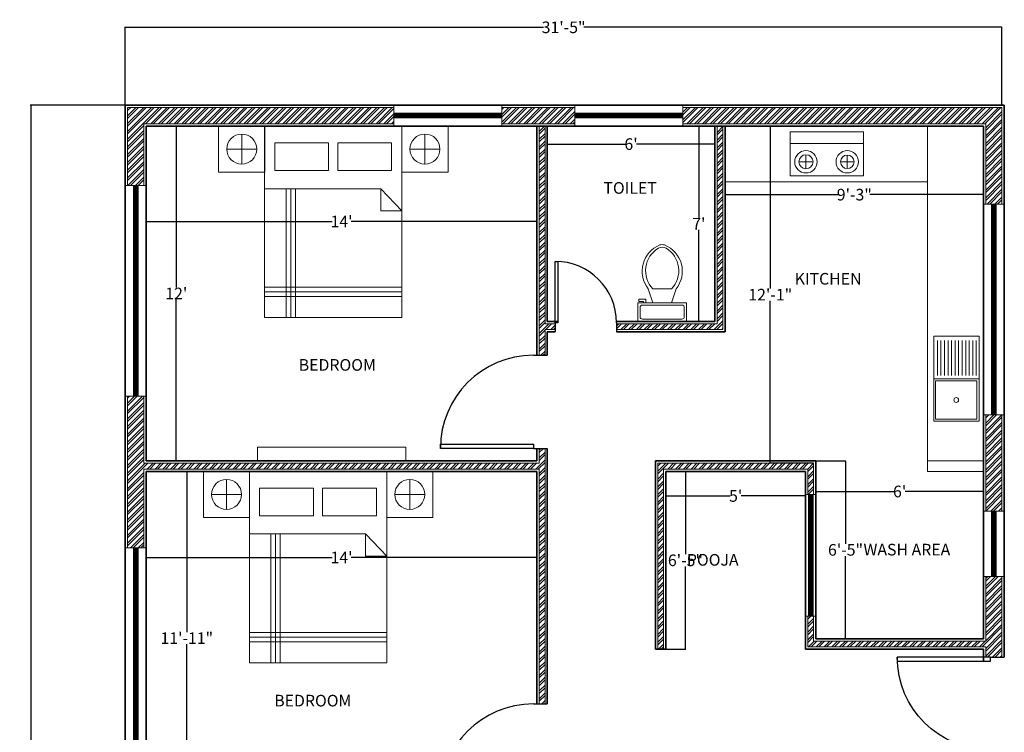
# Model space of a CAD drawing. Units: inches. Extents: x 210 to 633, y 286 to 1043.
# Tile 3 of 3: x 210 to 633, y 736 to 1043. Entities that reach past the tile are written whole.
import ezdxf

# ---------------------------------------------------------------- set-up
doc = ezdxf.new("R2010")
doc.units = ezdxf.units.IN
doc.header["$MEASUREMENT"] = 0
for name, color, linetype, lineweight in [('A-ANNO-DIMS', 170, 'Continuous', 18), ('A-AREA-IDEN', 7, 'Continuous', 25), ('A-DOOR', 4, 'Continuous', 25), ('A-EQPM', 210, 'Continuous', 18), ('A-FLOR-CBNT', 210, 'Continuous', 20), ('A-FLOR-FIXT', 210, 'Continuous', 18), ('A-FLOR-FIXT-PATT', 210, 'Continuous', 13), ('A-GLAZ-PATT', 130, 'Continuous', 13), ('A-WALL-PATT', 35, 'Continuous', 13), ('fur', 210, 'Continuous', 18), ('wall', 10, 'Continuous', 35), ('wind', 130, 'Continuous', 18)]:
    doc.layers.add(name, color=color, linetype=linetype, lineweight=lineweight)
doc.styles.get("Standard").update_dxf_attribs({"font": 'arial.ttf'})
doc.dimstyles.get("Standard").update_dxf_attribs({"dimtxt": 5, "dimasz": 0.18, "dimexe": 0.18, "dimexo": 0.0625, "dimgap": 0.09, "dimtad": 0, "dimtih": 1, "dimtoh": 1, "dimdec": 0, "dimzin": 0, "dimdsep": 46, "dimlunit": 4, "dimtxsty": 'Standard', "dimcen": 0.09, "dimadec": 0, "dimazin": 0, "dimtfac": 1, "dimtdec": 0, "dimtofl": 0, "dimtmove": 0, "dimatfit": 3, "dimfxl": 1, "dimtolj": 1, "dimtzin": 0, "dimarcsym": 0})

# ---------------------------------------------------------------- blocks, each defined once
blk = doc.blocks.new('*U2')
for p, q in [((0, 0), (0, -6)), ((40, 0), (40, -6))]:
    blk.add_line(p, q)
blk.add_lwpolyline([(0, 0), (0, 40), (1.75, 40), (1.75, 0)], close=True)
blk.add_arc((0, 0), 40, 0, 90)
blk = doc.blocks.new('*U4')
for p, q in [((9.5, -6), (9.5, -2)), ((-8, -8.5), (-8, -8)), ((-7, -8), (-7, -9.5)), ((-4, -8), (-6, -14)), ((4, -8), (6, -14)), ((-10, -8.5), (-8, -8.5)), ((-10, -9.5), (-10, -8.5)), ((-7, -9.5), (-10, -9.5)), ((4, -14), (-4, -14))]:
    blk.add_line(p, q)
blk.add_lwpolyline([(10.5, -8), (10.5, 0), (-10.5, 0), (-10.5, -8)], close=True)
for points in [[(-9.5, -2), (-9.5, -6)], [(8.5, -1), (-8.5, -1)], [(-8.5, -7), (8.5, -7)]]:
    blk.add_lwpolyline(points)
for centre, radius, start, end in [((-8.62, -1.88), 0.884, 81.8699, 188.1301), ((8.62, -1.88), 0.884, 351.8699, 98.1301), ((-8.62, -6.12), 0.884, 171.8699, 278.1301), ((8.62, -6.12), 0.884, 261.8699, 8.1301), ((3.52, -21.58), 12.17, 141.4691, 247.9714), ((4.2, -21.82), 11.33, 136.3677, 238.9468), ((-3.52, -21.58), 12.17, 292.0284, 38.5307), ((-4.2, -21.82), 11.33, 301.053, 43.6321), ((0, -27.88), 4, 245.7318, 294.2682), ((0, -29), 4, 254.8605, 285.1395)]:
    blk.add_arc(centre, radius, start, end)
blk = doc.blocks.new('*D9')
at = {"layer": 'A-ANNO-DIMS', "color": 0, "lineweight": -2, "transparency": 16777216}
for p, q in [((264.37, 996.96), (264.37, 955.79)), ((432.37, 996.96), (432.37, 955.79)), ((264.55, 955.97), (344.28, 955.97)), ((432.19, 955.97), (352.47, 955.97))]:
    blk.add_line(p, q, dxfattribs=at)
at = {"layer": 'A-ANNO-DIMS', "color": 0, "transparency": 16777216}
for points in [[(264.55, 956), (264.55, 955.94), (264.37, 955.97)], [(432.19, 956), (432.19, 955.94), (432.37, 955.97)]]:
    blk.add_solid(points, dxfattribs=at)
at = {"layer": 'Defpoints', "color": 0, "transparency": 16777216}
for p in [(264.37, 997.02), (432.37, 997.02), (432.37, 955.97)]:
    blk.add_point(p, dxfattribs=at)
at = {"layer": 'A-ANNO-DIMS', "color": 0, "transparency": 16777216, "insert": (348.37, 955.97), "char_height": 5, "attachment_point": 5}
blk.add_mtext("\\A1;14'", dxfattribs=at)
blk = doc.blocks.new('*D10')
at = {"layer": 'A-ANNO-DIMS', "color": 0, "lineweight": -2, "transparency": 16777216}
for p, q in [((264.44, 997.02), (277.51, 997.02)), ((277.33, 996.84), (277.33, 927.62)), ((277.33, 853.2), (277.33, 922.42)), ((264.44, 853.02), (277.51, 853.02))]:
    blk.add_line(p, q, dxfattribs=at)
at = {"layer": 'A-ANNO-DIMS', "color": 0, "transparency": 16777216}
for points in [[(277.3, 996.84), (277.36, 996.84), (277.33, 997.02)], [(277.3, 853.2), (277.36, 853.2), (277.33, 853.02)]]:
    blk.add_solid(points, dxfattribs=at)
at = {"layer": 'Defpoints', "color": 0, "transparency": 16777216}
for p in [(264.37, 997.02), (277.33, 997.02), (264.37, 853.02)]:
    blk.add_point(p, dxfattribs=at)
at = {"layer": 'A-ANNO-DIMS', "color": 0, "transparency": 16777216, "insert": (277.33, 925.02), "char_height": 5, "attachment_point": 5}
blk.add_mtext("\\A1;12'", dxfattribs=at)
blk = doc.blocks.new('*D11')
at = {"layer": 'A-ANNO-DIMS', "color": 0, "lineweight": -2, "transparency": 16777216}
for p, q in [((436.87, 996.96), (436.87, 989.09)), ((508.87, 996.96), (508.87, 989.09)), ((437.05, 989.27), (470.47, 989.27)), ((508.69, 989.27), (475.28, 989.27))]:
    blk.add_line(p, q, dxfattribs=at)
at = {"layer": 'A-ANNO-DIMS', "color": 0, "transparency": 16777216}
for points in [[(437.05, 989.3), (437.05, 989.24), (436.87, 989.27)], [(508.69, 989.3), (508.69, 989.24), (508.87, 989.27)]]:
    blk.add_solid(points, dxfattribs=at)
at = {"layer": 'Defpoints', "color": 0, "transparency": 16777216}
for p in [(436.87, 997.02), (508.87, 997.02), (508.87, 989.27)]:
    blk.add_point(p, dxfattribs=at)
at = {"layer": 'A-ANNO-DIMS', "color": 0, "transparency": 16777216, "insert": (472.87, 989.27), "char_height": 5, "attachment_point": 5}
blk.add_mtext("\\A1;6'", dxfattribs=at)
blk = doc.blocks.new('*D12')
at = {"layer": 'A-ANNO-DIMS', "color": 0, "lineweight": -2, "transparency": 16777216}
for p, q in [((508.81, 997.02), (501.82, 997.02)), ((502, 996.84), (502, 957.61)), ((502, 913.2), (502, 952.43)), ((508.81, 913.02), (501.82, 913.02))]:
    blk.add_line(p, q, dxfattribs=at)
at = {"layer": 'A-ANNO-DIMS', "color": 0, "transparency": 16777216}
for points in [[(501.97, 996.84), (502.03, 996.84), (502, 997.02)], [(501.97, 913.2), (502.03, 913.2), (502, 913.02)]]:
    blk.add_solid(points, dxfattribs=at)
at = {"layer": 'Defpoints', "color": 0, "transparency": 16777216}
for p in [(502, 997.02), (508.87, 997.02), (508.87, 913.02)]:
    blk.add_point(p, dxfattribs=at)
at = {"layer": 'A-ANNO-DIMS', "color": 0, "transparency": 16777216, "insert": (502, 955.02), "char_height": 5, "attachment_point": 5}
blk.add_mtext("\\A1;7'", dxfattribs=at)
blk = doc.blocks.new('*D13')
at = {"layer": 'A-ANNO-DIMS', "color": 0, "lineweight": -2, "transparency": 16777216}
for p, q in [((513.37, 996.96), (513.37, 967.35)), ((624.37, 996.96), (624.37, 967.35)), ((513.55, 967.53), (562.14, 967.53)), ((624.19, 967.53), (575.61, 967.53))]:
    blk.add_line(p, q, dxfattribs=at)
at = {"layer": 'A-ANNO-DIMS', "color": 0, "transparency": 16777216}
for points in [[(513.55, 967.56), (513.55, 967.5), (513.37, 967.53)], [(624.19, 967.56), (624.19, 967.5), (624.37, 967.53)]]:
    blk.add_solid(points, dxfattribs=at)
at = {"layer": 'Defpoints', "color": 0, "transparency": 16777216}
for p in [(513.37, 997.02), (624.37, 997.02), (624.37, 967.53)]:
    blk.add_point(p, dxfattribs=at)
at = {"layer": 'A-ANNO-DIMS', "color": 0, "transparency": 16777216, "insert": (568.87, 967.53), "char_height": 5, "attachment_point": 5}
blk.add_mtext('\\A1;9\'-3"', dxfattribs=at)
blk = doc.blocks.new('*D14')
at = {"layer": 'A-ANNO-DIMS', "color": 0, "lineweight": -2, "transparency": 16777216}
for p, q in [((551.31, 997.02), (532.55, 997.02)), ((532.73, 996.84), (532.73, 927.12)), ((532.73, 852.2), (532.73, 921.92)), ((551.31, 852.02), (532.55, 852.02))]:
    blk.add_line(p, q, dxfattribs=at)
at = {"layer": 'A-ANNO-DIMS', "color": 0, "transparency": 16777216}
for points in [[(532.7, 996.84), (532.76, 996.84), (532.73, 997.02)], [(532.7, 852.2), (532.76, 852.2), (532.73, 852.02)]]:
    blk.add_solid(points, dxfattribs=at)
at = {"layer": 'Defpoints', "color": 0, "transparency": 16777216}
for p in [(532.73, 997.02), (551.37, 997.02), (551.37, 852.02)]:
    blk.add_point(p, dxfattribs=at)
at = {"layer": 'A-ANNO-DIMS', "color": 0, "transparency": 16777216, "insert": (532.73, 924.52), "char_height": 5, "attachment_point": 5}
blk.add_mtext('\\A1;12\'-1"', dxfattribs=at)
blk = doc.blocks.new('*D15')
at = {"layer": 'A-ANNO-DIMS', "color": 0, "lineweight": -2, "transparency": 16777216}
for p, q in [((487.87, 848.46), (487.87, 837.78)), ((547.87, 848.46), (547.87, 837.78)), ((488.05, 837.96), (515.48, 837.96)), ((547.69, 837.96), (520.26, 837.96))]:
    blk.add_line(p, q, dxfattribs=at)
at = {"layer": 'A-ANNO-DIMS', "color": 0, "transparency": 16777216}
for points in [[(488.05, 837.99), (488.05, 837.93), (487.87, 837.96)], [(547.69, 837.99), (547.69, 837.93), (547.87, 837.96)]]:
    blk.add_solid(points, dxfattribs=at)
at = {"layer": 'Defpoints', "color": 0, "transparency": 16777216}
for p in [(487.87, 848.52), (547.87, 848.52), (547.87, 837.96)]:
    blk.add_point(p, dxfattribs=at)
at = {"layer": 'A-ANNO-DIMS', "color": 0, "transparency": 16777216, "insert": (517.87, 837.96), "char_height": 5, "attachment_point": 5}
blk.add_mtext("\\A1;5'", dxfattribs=at)
blk = doc.blocks.new('*D16')
at = {"layer": 'A-ANNO-DIMS', "color": 0, "lineweight": -2, "transparency": 16777216}
for p, q in [((487.94, 848.52), (496.43, 848.52)), ((496.25, 848.34), (496.25, 812.91)), ((496.25, 772.2), (496.25, 807.63)), ((487.94, 772.02), (496.43, 772.02))]:
    blk.add_line(p, q, dxfattribs=at)
at = {"layer": 'A-ANNO-DIMS', "color": 0, "transparency": 16777216}
for points in [[(496.22, 848.34), (496.28, 848.34), (496.25, 848.52)], [(496.22, 772.2), (496.28, 772.2), (496.25, 772.02)]]:
    blk.add_solid(points, dxfattribs=at)
at = {"layer": 'Defpoints', "color": 0, "transparency": 16777216}
for p in [(487.87, 848.52), (496.25, 848.52), (487.87, 772.02)]:
    blk.add_point(p, dxfattribs=at)
at = {"layer": 'A-ANNO-DIMS', "color": 0, "transparency": 16777216, "insert": (496.25, 810.27), "char_height": 5, "attachment_point": 5}
blk.add_mtext('\\A1;6\'-5"', dxfattribs=at)
blk = doc.blocks.new('*D17')
at = {"layer": 'A-ANNO-DIMS', "color": 0, "lineweight": -2, "transparency": 16777216}
for p, q in [((552.37, 852.96), (552.37, 839.69)), ((624.37, 852.03), (624.37, 839.69)), ((552.55, 839.87), (585.97, 839.87)), ((624.19, 839.87), (590.78, 839.87))]:
    blk.add_line(p, q, dxfattribs=at)
at = {"layer": 'A-ANNO-DIMS', "color": 0, "transparency": 16777216}
for points in [[(552.55, 839.9), (552.55, 839.84), (552.37, 839.87)], [(624.19, 839.9), (624.19, 839.84), (624.37, 839.87)]]:
    blk.add_solid(points, dxfattribs=at)
at = {"layer": 'Defpoints', "color": 0, "transparency": 16777216}
for p in [(552.37, 853.02), (624.37, 852.09), (624.37, 839.87)]:
    blk.add_point(p, dxfattribs=at)
at = {"layer": 'A-ANNO-DIMS', "color": 0, "transparency": 16777216, "insert": (588.37, 839.87), "char_height": 5, "attachment_point": 5}
blk.add_mtext("\\A1;6'", dxfattribs=at)
blk = doc.blocks.new('*D18')
at = {"layer": 'A-ANNO-DIMS', "color": 0, "lineweight": -2, "transparency": 16777216}
for p, q in [((552.44, 853.02), (565.28, 853.02)), ((565.1, 852.84), (565.1, 817.41)), ((565.1, 776.7), (565.1, 812.13)), ((552.44, 776.52), (565.28, 776.52))]:
    blk.add_line(p, q, dxfattribs=at)
at = {"layer": 'A-ANNO-DIMS', "color": 0, "transparency": 16777216}
for points in [[(565.07, 852.84), (565.13, 852.84), (565.1, 853.02)], [(565.07, 776.7), (565.13, 776.7), (565.1, 776.52)]]:
    blk.add_solid(points, dxfattribs=at)
at = {"layer": 'Defpoints', "color": 0, "transparency": 16777216}
for p in [(552.37, 853.02), (565.1, 853.02), (552.37, 776.52)]:
    blk.add_point(p, dxfattribs=at)
at = {"layer": 'A-ANNO-DIMS', "color": 0, "transparency": 16777216, "insert": (565.1, 814.77), "char_height": 5, "attachment_point": 5}
blk.add_mtext('\\A1;6\'-5"', dxfattribs=at)
blk = doc.blocks.new('*D19')
at = {"layer": 'A-ANNO-DIMS', "color": 0, "lineweight": -2, "transparency": 16777216}
for p, q in [((264.37, 848.46), (264.37, 811.29)), ((432.37, 848.46), (432.37, 811.29)), ((264.55, 811.47), (344.28, 811.47)), ((432.19, 811.47), (352.47, 811.47))]:
    blk.add_line(p, q, dxfattribs=at)
at = {"layer": 'A-ANNO-DIMS', "color": 0, "transparency": 16777216}
for points in [[(264.55, 811.5), (264.55, 811.44), (264.37, 811.47)], [(432.19, 811.5), (432.19, 811.44), (432.37, 811.47)]]:
    blk.add_solid(points, dxfattribs=at)
at = {"layer": 'Defpoints', "color": 0, "transparency": 16777216}
for p in [(264.37, 848.52), (432.37, 848.52), (432.37, 811.47)]:
    blk.add_point(p, dxfattribs=at)
at = {"layer": 'A-ANNO-DIMS', "color": 0, "transparency": 16777216, "insert": (348.37, 811.47), "char_height": 5, "attachment_point": 5}
blk.add_mtext("\\A1;14'", dxfattribs=at)
blk = doc.blocks.new('*D20')
at = {"layer": 'A-ANNO-DIMS', "color": 0, "lineweight": -2, "transparency": 16777216}
for p, q in [((264.44, 848.52), (282.01, 848.52)), ((281.83, 848.34), (281.83, 779.38)), ((281.83, 705.21), (281.83, 774.18)), ((264.44, 705.03), (282.01, 705.03))]:
    blk.add_line(p, q, dxfattribs=at)
at = {"layer": 'A-ANNO-DIMS', "color": 0, "transparency": 16777216}
for points in [[(281.8, 848.34), (281.86, 848.34), (281.83, 848.52)], [(281.8, 705.21), (281.86, 705.21), (281.83, 705.03)]]:
    blk.add_solid(points, dxfattribs=at)
at = {"layer": 'Defpoints', "color": 0, "transparency": 16777216}
for p in [(264.37, 848.52), (281.83, 848.52), (264.37, 705.03)]:
    blk.add_point(p, dxfattribs=at)
at = {"layer": 'A-ANNO-DIMS', "color": 0, "transparency": 16777216, "insert": (281.83, 776.78), "char_height": 5, "attachment_point": 5}
blk.add_mtext('\\A1;11\'-11"', dxfattribs=at)
blk = doc.blocks.new('*D36')
at = {"layer": 'A-ANNO-DIMS', "color": 0, "lineweight": -2, "transparency": 16777216}
for p, q in [((255.31, 1006.02), (214.53, 1006.02)), ((214.71, 1005.84), (214.71, 648.66)), ((214.71, 286.2), (214.71, 643.38)), ((255.31, 286.02), (214.53, 286.02))]:
    blk.add_line(p, q, dxfattribs=at)
at = {"layer": 'A-ANNO-DIMS', "color": 0, "transparency": 16777216}
for points in [[(214.68, 1005.84), (214.74, 1005.84), (214.71, 1006.02)], [(214.68, 286.2), (214.74, 286.2), (214.71, 286.02)]]:
    blk.add_solid(points, dxfattribs=at)
at = {"layer": 'Defpoints', "color": 0, "transparency": 16777216}
for p in [(214.71, 1006.02), (255.37, 1006.02), (255.37, 286.02)]:
    blk.add_point(p, dxfattribs=at)
at = {"layer": 'A-ANNO-DIMS', "color": 0, "transparency": 16777216, "insert": (214.71, 646.02), "char_height": 5, "attachment_point": 5}
blk.add_mtext("\\A1;60'", dxfattribs=at)
blk = doc.blocks.new('*D37')
at = {"layer": 'A-ANNO-DIMS', "color": 0, "lineweight": -2, "transparency": 16777216}
for p, q in [((255.37, 1006.08), (255.37, 1039.67)), ((255.55, 1039.49), (435.2, 1039.49)), ((632.19, 1039.49), (452.55, 1039.49)), ((632.37, 1006.08), (632.37, 1039.67))]:
    blk.add_line(p, q, dxfattribs=at)
at = {"layer": 'A-ANNO-DIMS', "color": 0, "transparency": 16777216}
for points in [[(255.55, 1039.52), (255.55, 1039.46), (255.37, 1039.49)], [(632.19, 1039.52), (632.19, 1039.46), (632.37, 1039.49)]]:
    blk.add_solid(points, dxfattribs=at)
at = {"layer": 'Defpoints', "color": 0, "transparency": 16777216}
for p in [(632.37, 1039.49), (255.37, 1006.02), (632.37, 1006.02)]:
    blk.add_point(p, dxfattribs=at)
at = {"layer": 'A-ANNO-DIMS', "color": 0, "transparency": 16777216, "insert": (443.87, 1039.49), "char_height": 5, "attachment_point": 5}
blk.add_mtext('\\A1;31\'-5"', dxfattribs=at)
blk = doc.blocks.new('BED-DOUBLE-WITH-NIGHTSTANDS')
for p, q in [((-9.81, -16.35), (-9.81, -3.45)), ((68.98, -16.35), (68.98, -3.45)), ((-16.26, -9.9), (-3.36, -9.9)), ((62.53, -9.9), (75.44, -9.9)), ((0, -26.92), (49.96, -26.92)), ((9.25, -26.92), (9.25, -82.32)), ((11.25, -26.92), (11.25, -82.32)), ((13.25, -26.92), (13.25, -82.32)), ((49.96, -26.92), (49.96, -36.42)), ((59.05, -36.42), (49.96, -26.92)), ((49.96, -36.42), (59.05, -36.42)), ((0, -69.31), (59.05, -69.31)), ((0, -71.31), (59.05, -71.31)), ((0, -73.31), (59.05, -73.31))]:
    blk.add_line(p, q)
for points in [[(0, 0), (59.05, 0), (59.05, -82.32), (0, -82.32)], [(-19.74, 0), (0.13, 0), (0.13, -19.81), (-19.74, -19.81)], [(59.05, 0), (78.92, 0), (78.92, -19.81), (59.05, -19.81)], [(4.4, -7.27), (27.55, -7.27), (27.55, -19.1), (4.4, -19.1)], [(31.46, -7.27), (54.61, -7.27), (54.61, -19.1), (31.46, -19.1)]]:
    blk.add_lwpolyline(points, close=True)
for centre in [(-9.81, -9.9), (68.98, -9.9)]:
    blk.add_circle(centre, 6.45)

msp = doc.modelspace()

# ---------------------------------------------------------------- hatches: boundary and pattern name
at = {"layer": 'A-FLOR-FIXT-PATT'}
h = msp.add_hatch(dxfattribs=at)
h.set_pattern_fill('ANSI31', color=256, scale=12.15317, angle=45, style=0)
h.paths.add_polyline_path([(604.26, 889.79), (621.52, 889.79), (621.52, 904.85), (604.26, 904.85)])
at = {"layer": 'A-GLAZ-PATT'}
h = msp.add_hatch(dxfattribs=at)
h.set_pattern_fill('ANSI31', color=256)
h.paths.add_polyline_path([(580.59, 368.5), (495.79, 368.5), (495.79, 366.5), (580.59, 366.5)])
h.paths.add_polyline_path([(629.87, 441.57), (627.87, 441.57), (627.87, 386.08), (629.87, 386.08)])
h.paths.add_polyline_path([(260.87, 537.72), (258.87, 537.72), (258.87, 447.09), (260.87, 447.09)])
h.paths.add_polyline_path([(260.87, 615.48), (258.87, 615.48), (258.87, 587.48), (260.87, 587.48)])
h.paths.add_polyline_path([(260.87, 685.1), (258.87, 685.1), (258.87, 657.11), (260.87, 657.11)])
h.paths.add_polyline_path([(629.87, 691.84), (627.87, 691.84), (627.87, 663.85), (629.87, 663.85)])
h.paths.add_polyline_path([(260.87, 815.6), (258.87, 815.6), (258.87, 724.96), (260.87, 724.96)])
h.paths.add_polyline_path([(629.87, 831.37), (627.87, 831.37), (627.87, 803.38), (629.87, 803.38)])
h.paths.add_polyline_path([(629.87, 963.44), (627.87, 963.44), (627.87, 872.81), (629.87, 872.81)])
h.paths.add_polyline_path([(495.13, 1002.52), (448.67, 1002.52), (448.67, 1000.52), (495.13, 1000.52)])
h.paths.add_polyline_path([(417.29, 1002.52), (370.83, 1002.52), (370.83, 1000.52), (417.29, 1000.52)])
h.paths.add_polyline_path([(260.87, 971.49), (258.87, 971.49), (258.87, 880.85), (260.87, 880.85)])
h = msp.add_hatch(dxfattribs=at)
h.set_pattern_fill('ANSI31', color=256)
h.paths.add_polyline_path([(551.12, 838.61), (549.12, 838.61), (549.12, 786.25), (551.12, 786.25)])
at = {"layer": 'A-WALL-PATT'}
h = msp.add_hatch(dxfattribs=at)
h.set_pattern_fill('ANSI32', color=256, scale=6.3)
h.paths.add_polyline_path([(370.83, 1005.02), (256.37, 1005.02), (256.37, 971.49), (263.37, 971.49), (263.37, 998.02), (370.83, 998.02)])
h.paths.add_polyline_path([(448.67, 1005.02), (417.29, 1005.02), (417.29, 998.02), (432.37, 998.02), (448.67, 998.02)])
h.paths.add_polyline_path([(632.37, 1005.02), (495.13, 1005.02), (495.13, 998.02), (508.87, 998.02), (625.37, 998.02), (625.37, 963.44), (632.37, 963.44)])
h.paths.add_polyline_path([(263.37, 849.52), (433.37, 849.52), (433.37, 748.51), (435.87, 748.51), (435.87, 849.52), (435.87, 858.43), (433.37, 858.43), (433.37, 852.02), (263.37, 852.02), (263.37, 880.85), (256.37, 880.85), (256.37, 815.6), (263.37, 815.6)])
h.paths.add_polyline_path([(263.37, 724.96), (256.37, 724.96), (256.37, 685.1), (263.37, 685.1)])
h.paths.add_polyline_path([(354.65, 703.52), (264.37, 703.52), (264.37, 701.02), (354.65, 701.02)])
h.paths.add_polyline_path([(263.37, 657.11), (256.37, 657.11), (256.37, 615.48), (263.37, 615.48)])
h = msp.add_hatch(dxfattribs=at)
h.set_pattern_fill('ANSI32', color=256, scale=6.3)
h.paths.add_polyline_path([(551.37, 786.25), (548.87, 786.25), (548.87, 773.02), (625.37, 773.02), (625.37, 768.63), (627.37, 768.63), (632.37, 768.63), (632.37, 803.38), (625.37, 803.38), (625.37, 775.52), (551.37, 775.52)])
h.paths.add_polyline_path([(435.87, 997.02), (433.37, 997.02), (433.37, 898.43), (435.87, 898.43), (435.87, 909.52), (440.28, 909.52), (440.28, 912.02), (435.87, 912.02)])
h.paths.add_polyline_path([(512.37, 997.02), (509.87, 997.02), (509.87, 912.02), (466.62, 912.02), (466.62, 909.52), (512.37, 909.52)])
h.paths.add_polyline_path([(435.87, 708.51), (433.37, 708.51), (433.37, 703.52), (381, 703.52), (381, 701.02), (435.87, 701.02)])
h.paths.add_polyline_path([(387.87, 700.02), (385.37, 700.02), (385.37, 639.02), (264.37, 639.02), (264.37, 636.52), (385.37, 636.52), (385.37, 574.52), (381, 574.52), (381, 572.02), (390.4, 572.02), (390.4, 574.43), (387.87, 574.43), (387.87, 635.52)])
h = msp.add_hatch(dxfattribs=at)
h.set_pattern_fill('ANSI32', color=256, scale=6.3)
h.paths.add_polyline_path([(486.87, 849.52), (526.87, 849.52), (548.87, 849.52), (548.87, 838.61), (551.37, 838.61), (551.37, 848.52), (551.37, 852.02), (531.37, 852.02), (484.37, 852.02), (484.37, 772.02), (486.87, 772.02), (486.87, 776.52)])
h.paths.add_polyline_path([(632.37, 872.81), (625.37, 872.81), (625.37, 831.37), (632.37, 831.37)])

# ---------------------------------------------------------------- linework, layer by layer
at = {"layer": 'A-EQPM'}
for p, q in [((541.25, 989.53), (572.84, 989.53)), ((548.09, 978.64), (548.09, 984.68)), ((565.85, 978.75), (565.85, 984.56)), ((545.07, 981.66), (551.11, 981.66)), ((562.95, 981.66), (568.76, 981.66))]:
    msp.add_line(p, q, dxfattribs=at)
msp.add_lwpolyline([(541.25, 994.59), (572.84, 994.59), (572.84, 975.56), (541.25, 975.56)], close=True, dxfattribs=at)
for centre, radius in [((548.09, 981.66), 4.82), ((548.09, 981.66), 3.02), ((565.85, 981.66), 4.82), ((565.85, 981.66), 2.91)]:
    msp.add_circle(centre, radius, dxfattribs=at)
at = {"layer": 'A-FLOR-CBNT'}
for p, q in [((513.37, 997.02), (513.37, 973.02)), ((600.37, 853.02), (600.37, 997.02)), ((513.37, 973.02), (593.09, 973.02)), ((593.09, 973.02), (600.37, 973.02)), ((624.37, 853.02), (600.37, 853.02)), ((600.37, 853.02), (600.37, 848.52)), ((600.37, 853.02), (624.37, 853.02)), ((624.37, 848.52), (600.37, 848.52)), ((600.37, 848.52), (624.37, 848.52))]:
    msp.add_line(p, q, dxfattribs=at)
at = {"layer": 'A-FLOR-FIXT'}
msp.add_line((603.08, 888.38), (622.61, 888.38), dxfattribs=at)
for points in [[(603.08, 870.14), (622.61, 870.14), (622.61, 906.61), (603.08, 906.61)], [(603.83, 871.04), (621.59, 871.04), (621.59, 887.41), (603.83, 887.41)]]:
    msp.add_lwpolyline(points, close=True, dxfattribs=at)
msp.add_circle((612.71, 879.22), 1.03, dxfattribs=at)
at = {"layer": 'A-WALL-PATT'}
for p, q in [((256.37, 1005.02), (370.83, 1005.02)), ((256.37, 1005.02), (256.37, 971.49)), ((417.29, 1005.02), (448.67, 1005.02)), ((495.13, 1005.02), (632.37, 1005.02)), ((632.37, 963.44), (632.37, 1005.02)), ((263.37, 998.02), (263.37, 971.49)), ((263.37, 998.02), (370.83, 998.02)), ((264.37, 998.02), (370.83, 998.02)), ((417.29, 998.02), (432.37, 998.02)), ((417.29, 998.02), (448.67, 998.02)), ((433.37, 997.02), (433.37, 898.43)), ((435.87, 997.02), (435.87, 912.02)), ((436.87, 998.02), (448.67, 998.02)), ((495.13, 998.02), (508.87, 998.02)), ((495.13, 998.02), (625.37, 998.02)), ((509.87, 997.02), (509.87, 912.02)), ((512.37, 997.02), (512.37, 909.52)), ((625.37, 963.44), (625.37, 998.02)), ((440.28, 912.02), (435.87, 912.02)), ((509.87, 912.02), (466.62, 912.02)), ((440.28, 909.52), (435.87, 909.52)), ((435.87, 909.52), (435.87, 898.43)), ((512.37, 909.52), (466.62, 909.52)), ((256.37, 880.85), (256.37, 815.6)), ((263.37, 880.85), (263.37, 852.02)), ((625.37, 831.37), (625.37, 872.81)), ((632.37, 831.37), (632.37, 872.81)), ((433.37, 858.43), (433.37, 852.02)), ((435.87, 858.43), (435.87, 849.52)), ((433.37, 852.02), (263.37, 852.02)), ((484.37, 772.02), (484.37, 852.02)), ((484.37, 852.02), (531.37, 852.02)), ((531.37, 852.02), (551.37, 852.02)), ((551.37, 848.52), (551.37, 852.02)), ((433.37, 849.52), (263.37, 849.52)), ((263.37, 849.52), (263.37, 815.6)), ((433.37, 748.51), (433.37, 849.52)), ((435.87, 748.51), (435.87, 849.52)), ((486.87, 776.52), (486.87, 849.52)), ((486.87, 849.52), (526.87, 849.52)), ((526.87, 849.52), (548.87, 849.52)), ((548.87, 849.52), (548.87, 838.61)), ((551.37, 848.52), (551.37, 838.61)), ((625.37, 775.52), (625.37, 803.38)), ((632.37, 768.63), (632.37, 803.38)), ((548.87, 786.25), (548.87, 773.02)), ((551.37, 786.25), (551.37, 775.52)), ((486.87, 776.52), (486.87, 772.02)), ((551.37, 775.52), (625.37, 775.52)), ((548.87, 773.02), (625.37, 773.02)), ((625.37, 768.63), (625.37, 773.02))]:
    msp.add_line(p, q, dxfattribs=at)
at = {"layer": 'fur'}
msp.add_lwpolyline([(312.28, 853.02), (376.07, 853.02), (376.07, 858.92), (312.28, 858.92)], close=True, dxfattribs=at)
at = {"layer": 'wall'}
for p, q in [((255.37, 1006.02), (633.37, 1006.02)), ((255.37, 1006.02), (255.37, 286.02)), ((255.37, 971.49), (255.37, 1006.02)), ((370.83, 1006.02), (255.37, 1006.02)), ((448.67, 1006.02), (417.29, 1006.02)), ((633.37, 1006.02), (495.13, 1006.02)), ((633.37, 768.63), (633.37, 1006.02)), ((633.37, 963.44), (633.37, 1006.02)), ((264.37, 997.02), (624.37, 997.02)), ((264.37, 997.02), (264.37, 853.02)), ((264.37, 997.02), (432.37, 997.02)), ((264.37, 971.49), (264.37, 997.02)), ((264.37, 997.02), (370.83, 997.02)), ((417.29, 997.02), (448.67, 997.02)), ((432.37, 997.02), (432.37, 898.43)), ((432.37, 997.02), (432.37, 898.43)), ((436.87, 997.02), (436.87, 913.02)), ((436.87, 997.02), (508.87, 997.02)), ((436.87, 913.02), (436.87, 997.02)), ((495.13, 997.02), (624.37, 997.02)), ((508.87, 997.02), (508.87, 913.02)), ((508.87, 997.02), (508.87, 913.02)), ((508.87, 997.02), (508.87, 913.02)), ((513.37, 997.02), (513.37, 908.52)), ((513.37, 997.02), (513.37, 908.52)), ((513.37, 908.52), (513.37, 997.02)), ((624.37, 997.02), (624.37, 963.44)), ((624.37, 776.52), (624.37, 997.02)), ((441.43, 913.02), (436.87, 913.02)), ((440.28, 913.02), (436.87, 913.02)), ((508.87, 913.02), (466.62, 913.02)), ((508.87, 913.02), (466.62, 913.02)), ((440.28, 908.52), (436.87, 908.52)), ((436.87, 898.43), (436.87, 908.52)), ((436.87, 908.52), (440.28, 908.52)), ((436.87, 908.52), (436.87, 898.43)), ((513.37, 908.52), (466.62, 908.52)), ((466.62, 908.52), (513.37, 908.52)), ((255.37, 880.85), (255.37, 815.6)), ((264.37, 853.02), (264.37, 880.85)), ((624.37, 831.37), (624.37, 872.81)), ((633.37, 872.81), (633.37, 831.37)), ((432.37, 858.43), (432.37, 853.02)), ((432.37, 853.02), (432.37, 858.43)), ((436.87, 858.43), (436.87, 848.52)), ((436.87, 748.51), (436.87, 858.43)), ((432.37, 853.02), (264.37, 853.02)), ((432.37, 853.02), (264.37, 853.02)), ((483.37, 772.02), (483.37, 853.02)), ((483.37, 853.02), (531.37, 853.02)), ((483.37, 772.02), (483.37, 853.02)), ((483.37, 853.02), (552.37, 853.02)), ((531.37, 853.02), (552.37, 853.02)), ((552.37, 848.52), (552.37, 853.02)), ((552.37, 853.02), (552.37, 838.61)), ((264.37, 848.52), (264.37, 704.52)), ((432.37, 848.52), (264.37, 848.52)), ((264.37, 815.6), (264.37, 848.52)), ((264.37, 848.52), (432.37, 848.52)), ((264.37, 848.52), (264.37, 427.02)), ((432.37, 748.51), (432.37, 848.52)), ((432.37, 848.52), (432.37, 748.51)), ((436.87, 748.51), (436.87, 848.52)), ((487.87, 776.52), (487.87, 848.52)), ((487.87, 848.52), (526.87, 848.52)), ((547.87, 848.52), (487.87, 848.52)), ((487.87, 848.52), (487.87, 772.02)), ((526.87, 848.52), (547.87, 848.52)), ((547.87, 848.52), (547.87, 776.52)), ((547.87, 838.61), (547.87, 848.52)), ((552.37, 848.52), (552.37, 776.52)), ((624.37, 848.52), (624.37, 776.52)), ((624.37, 803.38), (624.37, 776.52)), ((633.37, 768.63), (633.37, 803.38)), ((547.87, 786.25), (547.87, 772.02)), ((552.37, 776.52), (552.37, 786.25)), ((487.87, 776.52), (487.87, 772.02)), ((547.87, 776.52), (547.87, 772.02)), ((552.37, 776.52), (624.37, 776.52)), ((624.37, 776.52), (552.37, 776.52)), ((487.87, 772.02), (483.37, 772.02)), ((547.87, 772.02), (624.37, 772.02)), ((547.87, 772.02), (624.37, 772.02)), ((624.37, 772.02), (624.37, 766.88)), ((624.37, 766.88), (624.37, 772.02)), ((624.37, 772.02), (624.37, 768.63))]:
    msp.add_line(p, q, dxfattribs=at)
at = {"layer": 'wind'}
for p, q in [((370.83, 1002.52), (417.29, 1002.52)), ((370.83, 1000.52), (417.29, 1000.52)), ((448.67, 1002.52), (495.13, 1002.52)), ((448.67, 1000.52), (495.13, 1000.52)), ((258.87, 880.85), (258.87, 971.49)), ((260.87, 880.85), (260.87, 971.49)), ((627.87, 872.81), (627.87, 963.44)), ((629.87, 872.81), (629.87, 963.44)), ((549.12, 786.25), (549.12, 838.61)), ((549.12, 786.25), (549.12, 838.61)), ((551.12, 786.25), (551.12, 838.61)), ((627.87, 803.38), (627.87, 831.37)), ((629.87, 803.38), (629.87, 831.37)), ((258.87, 724.96), (258.87, 815.6)), ((258.87, 724.96), (258.87, 815.6)), ((260.87, 724.96), (260.87, 815.6))]:
    msp.add_line(p, q, dxfattribs=at)
for points in [[(417.29, 1006.02), (370.83, 1006.02), (370.83, 997.02), (417.29, 997.02)], [(495.13, 1006.02), (448.67, 1006.02), (448.67, 997.02), (495.13, 997.02)], [(264.37, 880.85), (255.37, 880.85), (255.37, 971.49), (264.37, 971.49)], [(633.37, 872.81), (624.37, 872.81), (624.37, 963.44), (633.37, 963.44)], [(547.87, 786.25), (552.37, 786.25), (552.37, 838.61), (547.87, 838.61)], [(633.37, 831.37), (624.37, 831.37), (624.37, 803.38), (633.37, 803.38)], [(264.37, 724.96), (255.37, 724.96), (255.37, 815.6), (264.37, 815.6)]]:
    msp.add_lwpolyline(points, close=True, dxfattribs=at)

# ---------------------------------------------------------------- block references
at = {"layer": 'A-DOOR', "xscale": 0.6586539344507552, "yscale": 0.6586539344507552, "zscale": 0.6586539344507552}
msp.add_blockref('*U2', (440.28, 912.47), dxfattribs=at)
at = {"layer": 'A-DOOR', "rotation": 90}
for p in [(430.87, 858.43), (430.87, 708.51)]:
    msp.add_blockref('*U2', p, dxfattribs=at)
at = {"layer": 'A-DOOR', "xscale": -1, "rotation": 90}
msp.add_blockref('*U2', (627.37, 768.63), dxfattribs=at)
at = {"layer": 'A-FLOR-FIXT', "xscale": -1, "rotation": 180}
msp.add_blockref('*U4', (486.27, 913.02), dxfattribs=at)
at = {"layer": 'fur'}
for p in [(315.27, 997.02), (308.74, 848.52)]:
    msp.add_blockref('BED-DOUBLE-WITH-NIGHTSTANDS', p, dxfattribs=at)

# ---------------------------------------------------------------- texts
at = {"layer": 'A-AREA-IDEN', "char_height": 5, "attachment_point": 1}
for s, insert in [('TOILET', (461, 972.91)), ('KITCHEN', (543.23, 933.85)), ('BEDROOM', (329.97, 896.81)), ('WASH AREA', (572.81, 817.38)), ('POOJA', (496.88, 812.97)), ('BEDROOM', (319.44, 752.43))]:
    msp.add_mtext_dynamic_manual_height_columns(s, width=1430.1061, gutter_width=25, heights=[0], dxfattribs=dict(at, insert=insert))

# ---------------------------------------------------------------- dimensions: what is measured, and where the dimension line sits
at = {"layer": 'A-ANNO-DIMS'}
for base, p1, p2, picture, middle in [((632.37, 1039.49), (255.37, 1006.02), (632.37, 1006.02), '*D37', (443.87, 1039.49)), ((432.37, 955.97), (264.37, 997.02), (432.37, 997.02), '*D9', (348.37, 955.97)), ((508.87, 989.27), (436.87, 997.02), (508.87, 997.02), '*D11', (472.87, 989.27)), ((624.37, 967.53), (513.37, 997.02), (624.37, 997.02), '*D13', (568.87, 967.53)), ((624.37, 839.87), (552.37, 853.02), (624.37, 852.09), '*D17', (588.37, 839.87)), ((432.37, 811.47), (264.37, 848.52), (432.37, 848.52), '*D19', (348.37, 811.47)), ((547.87, 837.96), (487.87, 848.52), (547.87, 848.52), '*D15', (517.87, 837.96))]:
    dim = msp.add_linear_dim(base=base, p1=p1, p2=p2, dimstyle='Standard', override={"dimclrd": 0, "dimclre": 0, "dimclrt": 0}, dxfattribs=at)
    dim.commit()
    dim.dimension.update_dxf_attribs({"geometry": picture, "text_midpoint": middle})
for base, p1, p2, picture, middle in [((214.71, 1006.02), (255.37, 286.02), (255.37, 1006.02), '*D36', (214.71, 646.02)), ((277.33, 997.02), (264.37, 853.02), (264.37, 997.02), '*D10', (277.33, 925.02)), ((532.73, 997.02), (551.37, 852.02), (551.37, 997.02), '*D14', (532.73, 924.52)), ((565.0993065, 853.02178869), (552.37354481, 776.52178869), (552.37354481, 853.02178869), '*D18', (565.0993065, 814.77178869)), ((281.83, 848.52), (264.37, 705.03), (264.37, 848.52), '*D20', (281.83, 776.78)), ((496.24890038, 848.52178869), (487.87354481, 772.02178869), (487.87354481, 848.52178869), '*D16', (496.24890038, 810.27178869))]:
    dim = msp.add_linear_dim(base=base, p1=p1, p2=p2, angle=90, dimstyle='Standard', override={"dimclrd": 0, "dimclre": 0, "dimclrt": 0}, dxfattribs=at)
    dim.commit()
    dim.dimension.update_dxf_attribs({"geometry": picture, "text_midpoint": middle})
dim = msp.add_aligned_dim(p1=(508.87, 913.02), p2=(508.87, 997.02), distance=6.87, dimstyle='Standard', override={"dimclrd": 0, "dimclre": 0, "dimclrt": 0}, dxfattribs=at)
dim.commit()
dim.dimension.update_dxf_attribs({"geometry": '*D12', "text_midpoint": (502, 955.02)})

doc.saveas('drawing.dxf')
